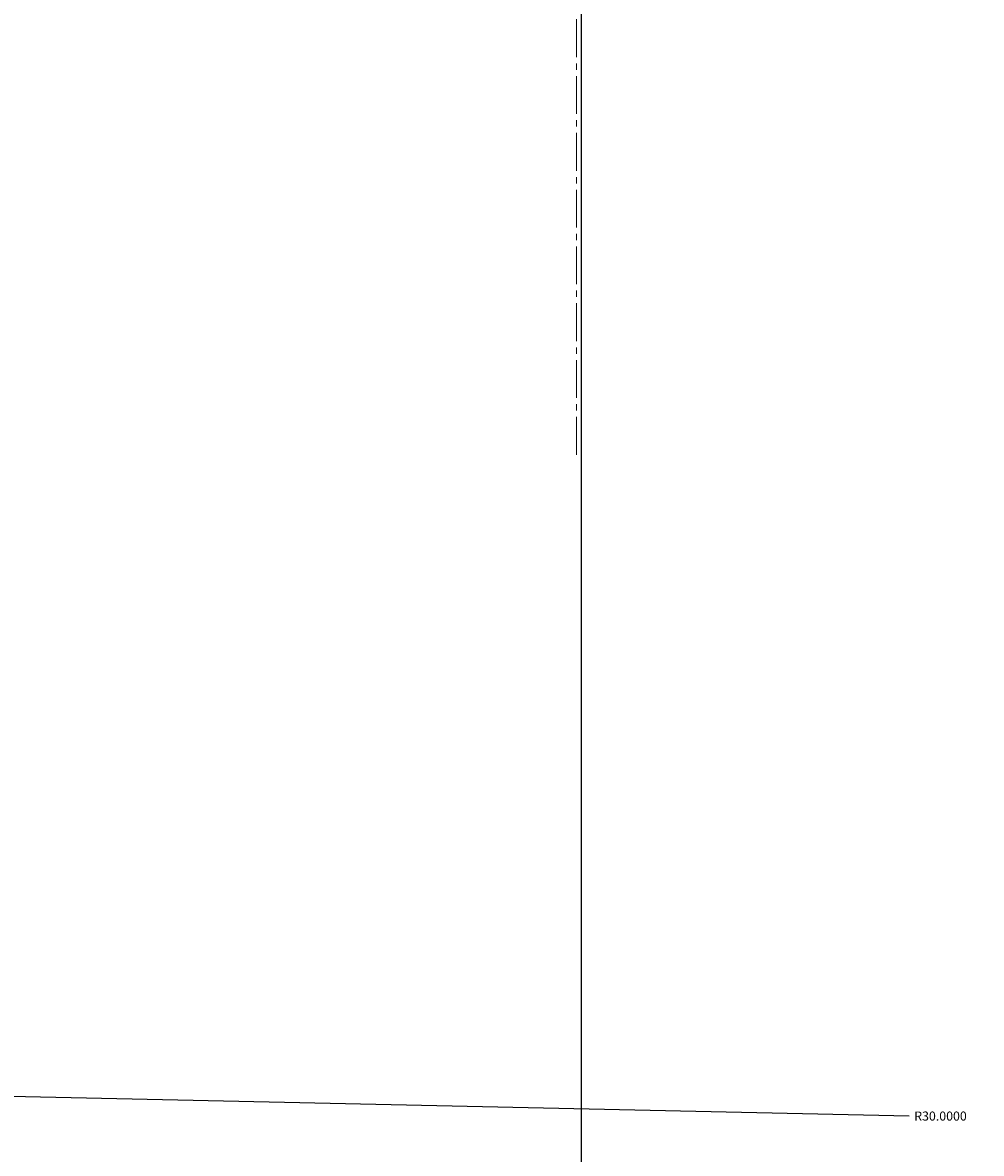
# Model space of a CAD drawing. Units: millimetres. Extents: x -60 to 113, y -37 to 126.
# Tile 9 of 17: x 0 to 19, y 48 to 70. Entities that reach past the tile are written whole.
import ezdxf

# ---------------------------------------------------------------- set-up
doc = ezdxf.new("R2010")
doc.units = ezdxf.units.MM
doc.header["$MEASUREMENT"] = 0
doc.linetypes.add('CENTER2', pattern=[1.125, 0.75, -0.125, 0.125, -0.125])
doc.layers.add('M-CNTR', color=4, linetype='CENTER2', lineweight=18)
doc.layers.add('M-DIMS', color=2, linetype='Continuous', lineweight=25)
doc.styles.get("Standard").update_dxf_attribs({"font": 'arial.ttf'})
doc.dimstyles.get("Standard").update_dxf_attribs({"dimtxt": 0.18, "dimasz": 0.18, "dimexe": 0.18, "dimexo": 0.0625, "dimgap": 0.09, "dimtad": 0, "dimtih": 1, "dimtoh": 1, "dimdec": 4, "dimzin": 0, "dimdsep": 46, "dimtxsty": 'Standard', "dimcen": 0.09, "dimadec": 0, "dimazin": 0, "dimtfac": 1, "dimtdec": 4, "dimtofl": 0, "dimtmove": 0, "dimatfit": 3, "dimfxl": 1, "dimtolj": 1, "dimtzin": 0, "dimarcsym": 0})

# ---------------------------------------------------------------- blocks, each defined once
blk = doc.blocks.new('*U1')
at = {"layer": 'M-CNTR', "color": 0, "transparency": 16777216}
blk.add_line((0, -27.12), (0, -5.4), dxfattribs=at)
blk = doc.blocks.new('*D7')
at = {"layer": 'Defpoints', "color": 0, "transparency": 16777216}
for p in [(48.606, 76.822), (-30.775, 49.351)]:
    blk.add_point(p, dxfattribs=at)
at = {"layer": 'M-DIMS', "color": 0, "lineweight": -2, "transparency": 16777216}
for p, q in [((37.821, 73.09), (48.435, 76.764)), ((37.641, 73.09), (37.821, 73.09))]:
    blk.add_line(p, q, dxfattribs=at)
at = {"layer": 'M-DIMS', "color": 0, "transparency": 16777216}
blk.add_solid([(48.426, 76.792), (48.445, 76.735), (48.606, 76.822)], dxfattribs=at)
at = {"layer": 'M-DIMS', "color": 0, "transparency": 16777216, "insert": (35.165, 73.09), "char_height": 0.18, "attachment_point": 5}
blk.add_mtext('\\A1;{\\H11.11111x;R84}', dxfattribs=at)
blk = doc.blocks.new('*D12')
at = {"layer": 'Defpoints', "color": 0, "transparency": 16777216}
for p in [(10.532, 88.533), (-58.719, 6.903), (11.329, 6.903)]:
    blk.add_point(p, dxfattribs=at)
at = {"layer": 'M-DIMS', "color": 0, "lineweight": -2, "transparency": 16777216}
for p, q in [((10.47, 88.533), (-58.899, 88.533)), ((-58.719, 88.353), (-58.719, 48.829)), ((-58.719, 7.083), (-58.719, 46.607)), ((11.267, 6.903), (-58.899, 6.903))]:
    blk.add_line(p, q, dxfattribs=at)
at = {"layer": 'M-DIMS', "color": 0, "transparency": 16777216}
for points in [[(-58.749, 88.353), (-58.689, 88.353), (-58.719, 88.533)], [(-58.749, 7.083), (-58.689, 7.083), (-58.719, 6.903)]]:
    blk.add_solid(points, dxfattribs=at)
at = {"layer": 'M-DIMS', "color": 0, "transparency": 16777216, "insert": (-58.719, 47.718), "char_height": 0.18, "attachment_point": 5}
blk.add_mtext('\\A1;{\\H11.11111x;82}', dxfattribs=at)
blk = doc.blocks.new('*D16')
at = {"layer": 'Defpoints', "color": 0, "transparency": 16777216}
for p in [(10.712, 88.533), (10.712, 88.533), (10.712, 6.442)]:
    blk.add_point(p, dxfattribs=at)
at = {"layer": 'M-DIMS', "color": 0, "lineweight": -2, "transparency": 16777216}
for p, q in [((10.712, 88.47), (10.712, 6.262)), ((10.712, 88.47), (10.712, 6.262)), ((10.532, 6.442), (10.352, 6.442)), ((10.892, 6.442), (11.072, 6.442))]:
    blk.add_line(p, q, dxfattribs=at)
at = {"layer": 'M-DIMS', "color": 0, "transparency": 16777216}
for points in [[(10.532, 6.472), (10.532, 6.412), (10.712, 6.442)], [(10.892, 6.472), (10.892, 6.412), (10.712, 6.442)]]:
    blk.add_solid(points, dxfattribs=at)
at = {"layer": 'M-DIMS', "color": 0, "transparency": 16777216, "insert": (11.536, 6.442), "char_height": 0.18, "attachment_point": 5}
blk.add_mtext('\\A1;0.0000', dxfattribs=at)
blk = doc.blocks.new('*D17')
at = {"layer": 'Defpoints', "color": 0, "transparency": 16777216}
for p in [(67.355, 124.823), (10.532, 88.533), (67.355, 6.442)]:
    blk.add_point(p, dxfattribs=at)
at = {"layer": 'M-DIMS', "color": 0, "lineweight": -2, "transparency": 16777216}
for p, q in [((10.532, 88.595), (10.532, 125.003)), ((10.712, 124.823), (37.422, 124.823)), ((67.175, 124.823), (40.465, 124.823)), ((67.355, 6.504), (67.355, 125.003))]:
    blk.add_line(p, q, dxfattribs=at)
at = {"layer": 'M-DIMS', "color": 0, "transparency": 16777216}
for points in [[(10.712, 124.853), (10.712, 124.793), (10.532, 124.823)], [(67.175, 124.853), (67.175, 124.793), (67.355, 124.823)]]:
    blk.add_solid(points, dxfattribs=at)
at = {"layer": 'M-DIMS', "color": 0, "transparency": 16777216, "insert": (38.944, 124.823), "char_height": 0.18, "attachment_point": 5}
blk.add_mtext('\\A1;{\\H11.11111x;56}', dxfattribs=at)
blk = doc.blocks.new('*D24')
at = {"layer": 'Defpoints', "color": 0, "transparency": 16777216}
for p in [(48.596, 76.851), (-30.775, 49.351)]:
    blk.add_point(p, dxfattribs=at)
at = {"layer": 'M-DIMS', "color": 0, "lineweight": -2, "transparency": 16777216}
for p, q in [((96.218, 93.35), (48.766, 76.909)), ((96.398, 93.35), (96.218, 93.35)), ((-30.865, 49.351), (-30.685, 49.351)), ((-30.775, 49.261), (-30.775, 49.441))]:
    blk.add_line(p, q, dxfattribs=at)
at = {"layer": 'M-DIMS', "color": 0, "transparency": 16777216}
blk.add_solid([(48.756, 76.938), (48.776, 76.881), (48.596, 76.851)], dxfattribs=at)
at = {"layer": 'M-DIMS', "color": 0, "transparency": 16777216, "insert": (97.018, 93.35), "char_height": 0.18, "attachment_point": 5}
blk.add_mtext('\\A1;R84.0000', dxfattribs=at)
blk = doc.blocks.new('*D25')
at = {"layer": 'Defpoints', "color": 0, "transparency": 16777216}
for p in [(-30.775, 49.351), (-0.782, 48.7)]:
    blk.add_point(p, dxfattribs=at)
at = {"layer": 'M-DIMS', "color": 0, "lineweight": -2, "transparency": 16777216}
for p, q in [((-30.865, 49.351), (-30.685, 49.351)), ((-30.775, 49.261), (-30.775, 49.441)), ((17.214, 48.309), (-0.602, 48.696))]:
    blk.add_line(p, q, dxfattribs=at)
at = {"layer": 'M-DIMS', "color": 0, "transparency": 16777216}
blk.add_solid([(-0.602, 48.726), (-0.603, 48.666), (-0.782, 48.7)], dxfattribs=at)
at = {"layer": 'M-DIMS', "color": 0, "transparency": 16777216, "insert": (17.833, 48.309), "char_height": 0.18, "attachment_point": 5}
blk.add_mtext('\\A1;R30.0000', dxfattribs=at)

msp = doc.modelspace()

# ---------------------------------------------------------------- block references
at = {"layer": 'M-CNTR'}
msp.add_blockref('*U1', (10.62227, 88.53289), dxfattribs=at)

# ---------------------------------------------------------------- dimensions: what is measured, and where the dimension line sits
at = {"layer": 'M-DIMS'}
dim = msp.add_linear_dim(base=(67.35481, 124.82251), p1=(10.53227, 88.53289), p2=(67.35481, 6.44179), text='{\\H11.11111x;56}', dimstyle='Standard', override={"dimclrd": 0, "dimclre": 0, "dimclrt": 0}, dxfattribs=at)
dim.commit()
dim.dimension.update_dxf_attribs({"geometry": '*D17', "text_midpoint": (38.94354, 124.82251)})
for mpoint, picture, middle in [((48.59582, 76.85052), '*D24', (97.01779, 93.35047)), ((-0.78224, 48.69961), '*D25', (17.21352, 48.30902))]:
    dim = msp.add_radius_dim(center=(-30.77517, 49.3506), mpoint=mpoint, dimstyle='Standard', override={"dimdec": 4, "dimlfac": 1, "dimrnd": 0, "dimzin": 0, "dimdsep": 46, "dimlunit": 2}, dxfattribs=at)
    dim.commit()
    dim.dimension.update_dxf_attribs({"geometry": picture, "text_midpoint": middle, "dimtype": 164})
dim = msp.add_linear_dim(base=(-58.71857, 6.9027), p1=(10.53227, 88.53289), p2=(11.32938, 6.9027), angle=90, text='{\\H11.11111x;82}', dimstyle='Standard', override={"dimclrd": 0, "dimclre": 0, "dimclrt": 0}, dxfattribs=at)
dim.commit()
dim.dimension.update_dxf_attribs({"geometry": '*D12', "text_midpoint": (-58.71857, 47.71779)})
dim = msp.add_linear_dim(base=(10.712269814, 6.441792179), p1=(10.712269814, 88.5328900903), p2=(10.712269814, 88.5328900903), dimstyle='Standard', override={"dimclrd": 0, "dimclre": 0, "dimclrt": 0}, dxfattribs=at)
dim.commit()
dim.dimension.update_dxf_attribs({"geometry": '*D16', "text_midpoint": (11.5355917785, 6.441792179)})
dim = msp.add_radius_dim(center=(-30.77517, 49.3506), mpoint=(48.60556, 76.82239), text='{\\H11.11111x;R84}', dimstyle='Standard', override={"dimclrd": 0, "dimclre": 0, "dimclrt": 0}, dxfattribs=at)
dim.commit()
dim.dimension.update_dxf_attribs({"geometry": '*D7', "text_midpoint": (35.16548, 73.09007), "dimtype": 164})

doc.saveas('drawing.dxf')
